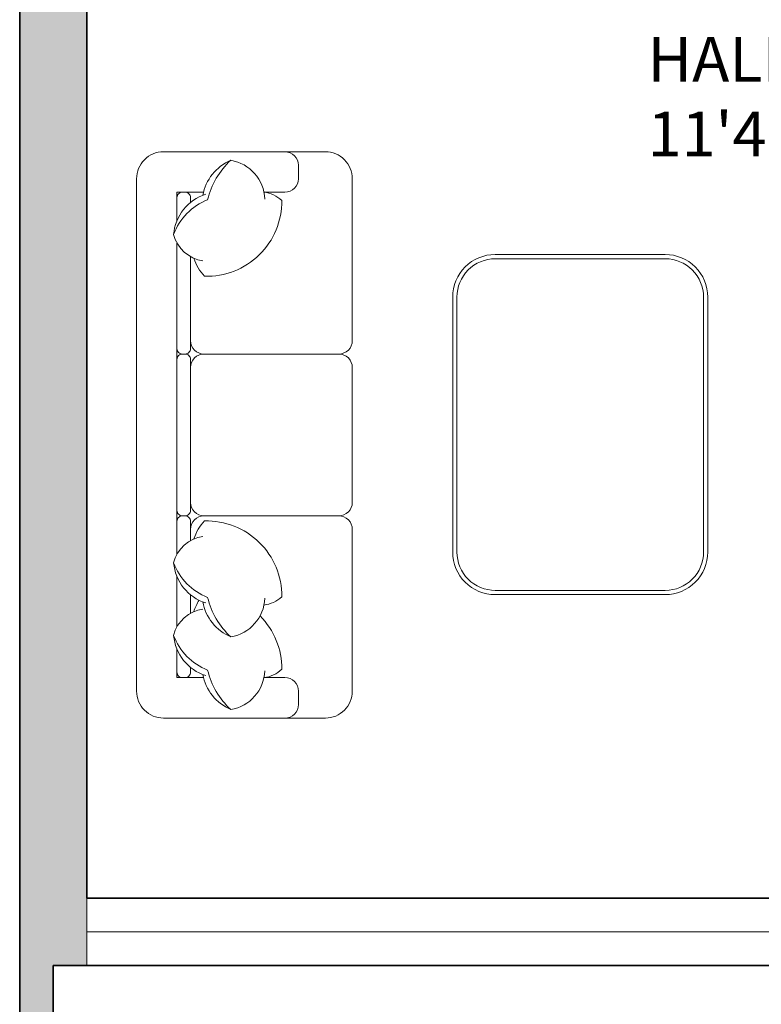
# Model space of a CAD drawing. Units: inches. Extents: x -5 to 366, y -496 to 54.
# Tile 3 of 10: x 22 to 121, y -337 to -205. Entities that reach past the tile are written whole.
import ezdxf

# ---------------------------------------------------------------- set-up
doc = ezdxf.new("R2010")
doc.units = ezdxf.units.IN
doc.header["$MEASUREMENT"] = 0
for name, color, linetype, lineweight in [('A-AREA-IDEN', 7, 'Continuous', 25), ('A-FURN', 8, 'Continuous', 18), ('A-GLAZ', 4, 'Continuous', 18), ('A-WALL', 7, 'Continuous', 35), ('A-WALL-PATT', 252, 'Continuous', 13)]:
    doc.layers.add(name, color=color, linetype=linetype, lineweight=lineweight)
doc.styles.get("Standard").update_dxf_attribs({"font": 'arial.ttf'})

msp = doc.modelspace()

# ---------------------------------------------------------------- hatches: boundary and pattern name
at = {"layer": 'A-WALL-PATT'}
h = msp.add_hatch(color=256, dxfattribs=at)
h.dxf.hatch_style = 1
h.paths.add_polyline_path([(324.93, 26.52), (21.93, 26.52), (21.93, -456.98), (26.43, -456.98), (26.43, -331.98), (30.93, -331.98), (30.93, -322.98), (30.93, -106.98), (110.93, -106.98), (110.93, -104.73), (110.93, -102.48), (30.93, -102.48), (30.93, 17.52), (138.93, 17.52), (141.18, 17.52), (143.43, 17.52), (183.43, 17.52), (187.93, 17.52), (315.93, 17.52), (315.93, -102.48), (315.93, -106.98), (315.93, -255.48), (171.93, -255.48), (171.93, -155.84), (167.43, -155.84), (167.43, -291.98), (171.93, -291.98), (171.93, -259.98), (315.93, -259.98), (315.93, -375.98), (297.93, -375.98), (297.93, -380.48), (315.93, -380.48), (315.93, -452.48), (315.93, -456.98), (324.93, -456.98)])
h.paths.add_polyline_path([(143.43, -18.48), (143.43, -13.98), (138.93, -13.98), (138.93, -106.98), (187.93, -106.98), (187.93, -102.48), (143.43, -102.48)], flags=17)

# ---------------------------------------------------------------- linework, layer by layer
at = {"layer": 'A-FURN', "ltscale": 0.03}
for points in [[(62.84, -223.05, -0.414214), (66.45, -226.66), (66.45, -248.32, -0.414214), (64.64, -250.12, -0.414214), (66.45, -251.93), (66.45, -269.98, -0.414214), (64.64, -271.78, -0.414214), (66.45, -273.59), (66.45, -295.25, -0.414214), (62.84, -298.86), (41.18, -298.86, -0.414214), (37.57, -295.25), (37.57, -226.66, -0.414214), (41.18, -223.05)], [(85.57, -236.8), (108.33, -236.8, -0.414214), (114.02, -242.49), (114.02, -276.64, -0.414214), (108.33, -282.33), (85.57, -282.33, -0.414214), (79.88, -276.64), (79.88, -242.49, -0.414214)], [(85.57, -237.37), (108.33, -237.37, -0.414214), (113.45, -242.49), (113.45, -276.64, -0.414214), (108.33, -281.76), (85.57, -281.76, -0.414214), (80.45, -276.64), (80.45, -242.49, -0.414214)]]:
    msp.add_lwpolyline(points, format="xyb", close=True, dxfattribs=at)
at = {"layer": 'A-FURN'}
for points in [[(57.42, -223.05, -0.414214), (59.23, -224.85), (59.23, -226.66, -0.414214), (57.42, -228.46), (54.62, -228.46)], [(50.18, -224.19, 0.14773), (47.08, -229.47, 0.213343), (42.53, -234.13, 0.178662)], [(54.73, -229.37, 0.356772), (50.18, -224.19, 0.249542), (46.43, -228.88, -9.61688)], [(46.83, -228.74, 0.306663), (42.53, -234.13, 0.30633), (46.46, -237.64, -0.872847)], [(44.79, -229.84), (44.79, -229.18, 0.414214), (44.06, -228.46), (43.7, -228.46, 0.414214), (42.98, -229.18)], [(42.98, -229.18), (42.98, -232.26, 0.414214)], [(54.62, -228.46, -0.165541), (57.01, -229.57, -0.425989), (46.67, -239.71, -0.121523), (45.24, -237.3, 7.115464)], [(42.98, -235.26), (42.98, -249.4, 0.414214), (43.7, -250.12), (44.06, -250.12, 0.414214), (44.79, -249.4), (44.79, -237.08, 0.414214)], [(44.79, -248.32, 0.414214), (46.59, -250.12), (64.64, -250.12, 0.414214)], [(44.79, -251.93, -0.414214), (46.59, -250.12)], [(44.79, -269.98, 0.414214), (46.59, -271.78)], [(42.98, -276.92), (42.98, -272.51, -0.414214), (43.7, -271.78), (44.06, -271.78, -0.414214), (44.79, -272.51), (44.79, -275.1, -0.414214)], [(44.79, -273.59, -0.414214), (46.59, -271.78), (64.64, -271.78, -0.414214)], [(54.62, -283.72, 0.165541), (57.01, -282.61, 0.425989), (46.67, -272.47, 0.121523), (45.24, -274.88, -7.115464)], [(46.83, -283.44, -0.306663), (42.53, -278.06, -0.30633), (46.46, -274.54, 0.872847)], [(50.18, -287.99, -0.14773), (47.08, -282.71, -0.213343), (42.53, -278.06, -0.178662)], [(42.98, -286.64), (42.98, -279.92, -0.414214)], [(44.79, -282.34), (44.79, -284.83, -0.414214)], [(45.95, -283.09, 0.071865), (45.24, -284.6, -7.115464)], [(54.73, -282.81, -0.356772), (50.18, -287.99, -0.249542), (46.43, -283.3, 9.61688)], [(46.83, -293.16, -0.306663), (42.53, -287.78, -0.30633), (46.46, -284.26, 0.872847)], [(54.62, -293.45, 0.165541), (57.01, -292.33, 0.200231), (54.1, -285.17, 0.121523)], [(50.18, -297.71, -0.14773), (47.08, -292.44, -0.213343), (42.53, -287.78, -0.178662)], [(42.98, -289.65), (42.98, -293.44), (46.53, -293.44, -0.414214)], [(42.98, -292.72), (42.98, -289.65, -0.414214)], [(44.79, -292.07), (44.79, -292.72, -0.414214), (44.06, -293.44), (43.7, -293.44, -0.414214), (42.98, -292.72)], [(54.73, -292.54, -0.356772), (50.18, -297.71, -0.249542), (46.43, -293.02, 9.61688)], [(54.62, -293.44), (57.42, -293.44, -0.414214), (59.23, -295.25), (59.23, -297.05, -0.414214), (57.42, -298.86)]]:
    msp.add_lwpolyline(points, format="xyb", dxfattribs=at)
for points in [[(46.53, -228.46), (42.98, -228.46), (42.98, -232.26)], [(42.98, -235.26), (42.98, -276.92)], [(42.98, -279.92), (42.98, -286.64)]]:
    msp.add_lwpolyline(points, dxfattribs=at)
msp.add_lwpolyline([(42.98, -271.06), (42.98, -250.84, -0.414214), (43.7, -250.12), (44.06, -250.12, -0.414214), (44.79, -250.84), (44.79, -271.06, -0.414214), (44.06, -271.78), (43.7, -271.78, -0.414214)], format="xyb", close=True, dxfattribs=at)
at = {"layer": 'A-GLAZ'}
for p, q in [((30.93, -322.98), (30.93, -331.98)), ((30.93, -327.48), (123.64, -327.48))]:
    msp.add_line(p, q, dxfattribs=at)
at = {"layer": 'A-WALL'}
for p, q in [((21.93, 26.52), (21.93, -456.98)), ((30.93, -106.98), (30.93, -322.98)), ((30.93, -322.98), (139.43, -322.98)), ((26.43, -331.98), (139.43, -331.98)), ((26.43, -331.98), (26.43, -456.98))]:
    msp.add_line(p, q, dxfattribs=at)

# ---------------------------------------------------------------- texts
at = {"layer": 'A-AREA-IDEN', "insert": (105.97, -207.67), "char_height": 6, "attachment_point": 1}
msp.add_mtext('HALL\\P11\'4"X18\'0"', dxfattribs=at)

doc.saveas('drawing.dxf')
